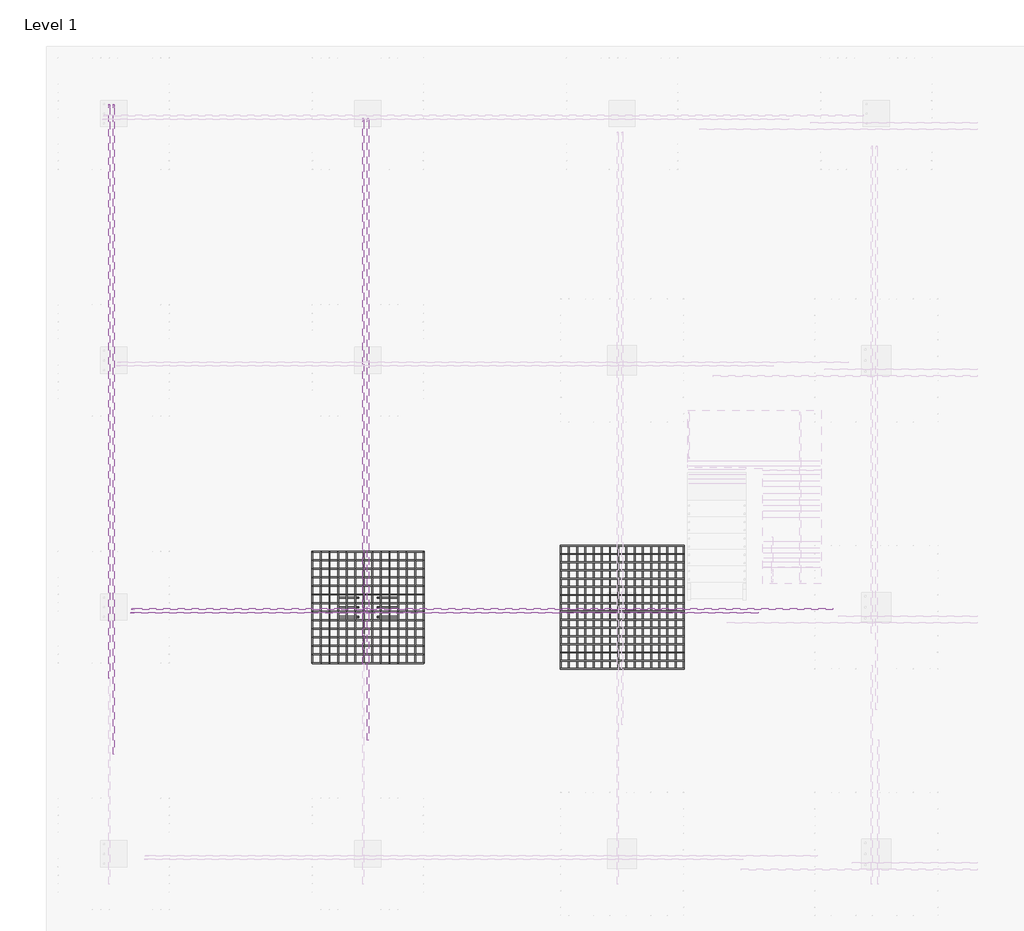
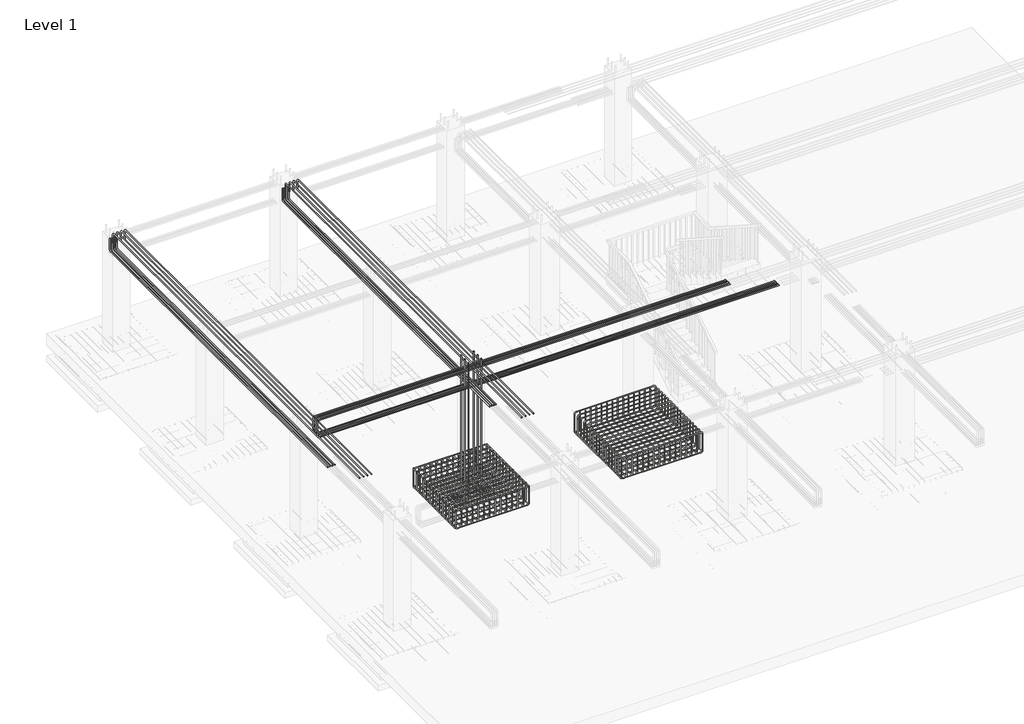
# One storey, part 9 of 17: 21 reinforcing bars.
"""IFC4 building model written with IfcOpenShell, lengths in millimetres."""

from ifc_helpers import new_model, si_unit, point, frame, origin, place, context, project, spatial, polyline, circle_curve, trimmed, segment, composite_curve, source, transform, mapped, element, save
from ifc_brep_helpers import swept_disk

model = new_model("IFC4")

# Units and contexts
model_context = context("Model", 3, world=origin())
ifc_project = project(units=[si_unit("LENGTHUNIT", "METRE", prefix="MILLI")], contexts=[model_context])

# Site, building, storey
site = spatial("IfcSite", under=ifc_project)
building = spatial("IfcBuilding", under=site)
storey = spatial("IfcBuildingStorey", under=building, Name="Level 1", Elevation=0.0)

# Reinforcing bars
placement = place(None, origin())
reinforcing_bar_shape = source(origin(), model_context, "Body", "SolidModel", [
    swept_disk(composite_curve([segment(polyline([(-9341.3632003, 4853.009457, -40.0), (-9341.3632003, 4853.009457, -504.0)]), True, "CONTINUOUS"), segment(trimmed(circle_curve(frame((-9293.3632003, 4853.009457, -504.0), z_axis=(0.0, -1.0, 0.0), x_axis=(-48.0, 0.0, 0.0)), 48.0), [point((-9341.3632003, 4853.009457, -504.0))], [point((-9293.3632003, 4853.009457, -552.0))], True, "CARTESIAN"), True, "CONTINUOUS"), segment(polyline([(-9293.3632003, 4853.009457, -552.0), (-7485.3632003, 4853.009457, -552.0)]), True, "CONTINUOUS"), segment(trimmed(circle_curve(frame((-7485.3632003, 4853.009457, -504.0), z_axis=(0.0, -1.0, 0.0), x_axis=(0.0, 0.0, -48.0)), 48.0), [point((-7485.3632003, 4853.009457, -552.0))], [point((-7437.3632003, 4853.009457, -504.0))], True, "CARTESIAN"), True, "CONTINUOUS"), segment(polyline([(-7437.3632003, 4853.009457, -504.0), (-7437.3632003, 4853.009457, -40.0)]), True, "CONTINUOUS")], self_intersect=False), 8.0),
])
element("IfcReinforcingBar", 1, at=placement, inside=storey, context=model_context, shape_type="MappedRepresentation", body=[
    mapped(reinforcing_bar_shape, transform((0.0, 0.0, 0.0), x_axis=(1.0, 0.0, 0.0), y_axis=(0.0, 1.0, 0.0), z_axis=(0.0, 0.0, 1.0))),
    mapped(reinforcing_bar_shape, transform((0.0, -146.4615385, 0.0), x_axis=(1.0, 0.0, 0.0), y_axis=(0.0, 1.0, 0.0), z_axis=(0.0, 0.0, 1.0))),
    mapped(reinforcing_bar_shape, transform((0.0, -292.9230769, 0.0), x_axis=(1.0, 0.0, 0.0), y_axis=(0.0, 1.0, 0.0), z_axis=(0.0, 0.0, 1.0))),
    mapped(reinforcing_bar_shape, transform((0.0, -439.3846154, 0.0), x_axis=(1.0, 0.0, 0.0), y_axis=(0.0, 1.0, 0.0), z_axis=(0.0, 0.0, 1.0))),
    mapped(reinforcing_bar_shape, transform((0.0, -585.8461538, 0.0), x_axis=(1.0, 0.0, 0.0), y_axis=(0.0, 1.0, 0.0), z_axis=(0.0, 0.0, 1.0))),
    mapped(reinforcing_bar_shape, transform((0.0, -732.3076923, 0.0), x_axis=(1.0, 0.0, 0.0), y_axis=(0.0, 1.0, 0.0), z_axis=(0.0, 0.0, 1.0))),
    mapped(reinforcing_bar_shape, transform((0.0, -878.7692308, 0.0), x_axis=(1.0, 0.0, 0.0), y_axis=(0.0, 1.0, 0.0), z_axis=(0.0, 0.0, 1.0))),
    mapped(reinforcing_bar_shape, transform((0.0, -1025.2307692, 0.0), x_axis=(1.0, 0.0, 0.0), y_axis=(0.0, 1.0, 0.0), z_axis=(0.0, 0.0, 1.0))),
    mapped(reinforcing_bar_shape, transform((0.0, -1171.6923077, 0.0), x_axis=(1.0, 0.0, 0.0), y_axis=(0.0, 1.0, 0.0), z_axis=(0.0, 0.0, 1.0))),
    mapped(reinforcing_bar_shape, transform((0.0, -1318.1538462, 0.0), x_axis=(1.0, 0.0, 0.0), y_axis=(0.0, 1.0, 0.0), z_axis=(0.0, 0.0, 1.0))),
    mapped(reinforcing_bar_shape, transform((0.0, -1464.6153846, 0.0), x_axis=(1.0, 0.0, 0.0), y_axis=(0.0, 1.0, 0.0), z_axis=(0.0, 0.0, 1.0))),
    mapped(reinforcing_bar_shape, transform((0.0, -1611.0769231, 0.0), x_axis=(1.0, 0.0, 0.0), y_axis=(0.0, 1.0, 0.0), z_axis=(0.0, 0.0, 1.0))),
    mapped(reinforcing_bar_shape, transform((0.0, -1757.5384615, 0.0), x_axis=(1.0, 0.0, 0.0), y_axis=(0.0, 1.0, 0.0), z_axis=(0.0, 0.0, 1.0))),
    mapped(reinforcing_bar_shape, transform((0.0, -1904.0, 0.0), x_axis=(1.0, 0.0, 0.0), y_axis=(0.0, 1.0, 0.0), z_axis=(0.0, 0.0, 1.0))),
])
reinforcing_bar_2_shape = source(origin(), model_context, "Body", "SolidModel", [
    swept_disk(composite_curve([segment(polyline([(-9341.3632003, 2949.009457, -504.0), (-9341.3632003, 2949.009457, -96.0)]), True, "CONTINUOUS"), segment(trimmed(circle_curve(frame((-9293.3632003, 2949.009457, -96.0), z_axis=(0.0, 1.0, 0.0), x_axis=(-48.0, 0.0, 0.0)), 48.0), [point((-9341.3632003, 2949.009457, -96.0))], [point((-9293.3632003, 2949.009457, -48.0))], True, "CARTESIAN"), True, "CONTINUOUS"), segment(polyline([(-9293.3632003, 2949.009457, -48.0), (-7485.3632003, 2949.009457, -48.0)]), True, "CONTINUOUS"), segment(trimmed(circle_curve(frame((-7485.3632003, 2949.009457, -96.0), z_axis=(0.0, 1.0, 0.0), x_axis=(0.0, 0.0, 48.0)), 48.0), [point((-7485.3632003, 2949.009457, -48.0))], [point((-7437.3632003, 2949.009457, -96.0))], True, "CARTESIAN"), True, "CONTINUOUS"), segment(polyline([(-7437.3632003, 2949.009457, -96.0), (-7437.3632003, 2949.009457, -504.0)]), True, "CONTINUOUS")], self_intersect=False), 8.0),
])
element("IfcReinforcingBar", 2, at=placement, inside=storey, context=model_context, shape_type="MappedRepresentation", body=[
    mapped(reinforcing_bar_2_shape, transform((0.0, 0.0, 0.0), x_axis=(1.0, 0.0, 0.0), y_axis=(0.0, 1.0, 0.0), z_axis=(0.0, 0.0, 1.0))),
    mapped(reinforcing_bar_2_shape, transform((0.0, 146.4615385, 0.0), x_axis=(1.0, 0.0, 0.0), y_axis=(0.0, 1.0, 0.0), z_axis=(0.0, 0.0, 1.0))),
    mapped(reinforcing_bar_2_shape, transform((0.0, 292.9230769, 0.0), x_axis=(1.0, 0.0, 0.0), y_axis=(0.0, 1.0, 0.0), z_axis=(0.0, 0.0, 1.0))),
    mapped(reinforcing_bar_2_shape, transform((0.0, 439.3846154, 0.0), x_axis=(1.0, 0.0, 0.0), y_axis=(0.0, 1.0, 0.0), z_axis=(0.0, 0.0, 1.0))),
    mapped(reinforcing_bar_2_shape, transform((0.0, 585.8461538, 0.0), x_axis=(1.0, 0.0, 0.0), y_axis=(0.0, 1.0, 0.0), z_axis=(0.0, 0.0, 1.0))),
    mapped(reinforcing_bar_2_shape, transform((0.0, 732.3076923, 0.0), x_axis=(1.0, 0.0, 0.0), y_axis=(0.0, 1.0, 0.0), z_axis=(0.0, 0.0, 1.0))),
    mapped(reinforcing_bar_2_shape, transform((0.0, 878.7692308, 0.0), x_axis=(1.0, 0.0, 0.0), y_axis=(0.0, 1.0, 0.0), z_axis=(0.0, 0.0, 1.0))),
    mapped(reinforcing_bar_2_shape, transform((0.0, 1025.2307692, 0.0), x_axis=(1.0, 0.0, 0.0), y_axis=(0.0, 1.0, 0.0), z_axis=(0.0, 0.0, 1.0))),
    mapped(reinforcing_bar_2_shape, transform((0.0, 1171.6923077, 0.0), x_axis=(1.0, 0.0, 0.0), y_axis=(0.0, 1.0, 0.0), z_axis=(0.0, 0.0, 1.0))),
    mapped(reinforcing_bar_2_shape, transform((0.0, 1318.1538462, 0.0), x_axis=(1.0, 0.0, 0.0), y_axis=(0.0, 1.0, 0.0), z_axis=(0.0, 0.0, 1.0))),
    mapped(reinforcing_bar_2_shape, transform((0.0, 1464.6153846, 0.0), x_axis=(1.0, 0.0, 0.0), y_axis=(0.0, 1.0, 0.0), z_axis=(0.0, 0.0, 1.0))),
    mapped(reinforcing_bar_2_shape, transform((0.0, 1611.0769231, 0.0), x_axis=(1.0, 0.0, 0.0), y_axis=(0.0, 1.0, 0.0), z_axis=(0.0, 0.0, 1.0))),
    mapped(reinforcing_bar_2_shape, transform((0.0, 1757.5384615, 0.0), x_axis=(1.0, 0.0, 0.0), y_axis=(0.0, 1.0, 0.0), z_axis=(0.0, 0.0, 1.0))),
    mapped(reinforcing_bar_2_shape, transform((0.0, 1904.0, 0.0), x_axis=(1.0, 0.0, 0.0), y_axis=(0.0, 1.0, 0.0), z_axis=(0.0, 0.0, 1.0))),
])
reinforcing_bar_3_shape = source(origin(), model_context, "Body", "SolidModel", [
    swept_disk(composite_curve([segment(polyline([(-7437.3632003, 4853.009457, -96.0), (-7437.3632003, 4853.009457, -504.0)]), True, "CONTINUOUS"), segment(trimmed(circle_curve(frame((-7437.3632003, 4805.009457, -504.0), z_axis=(-1.0, 0.0, 0.0), x_axis=(0.0, 48.0, 0.0)), 48.0), [point((-7437.3632003, 4853.009457, -504.0))], [point((-7437.3632003, 4805.009457, -552.0))], True, "CARTESIAN"), True, "CONTINUOUS"), segment(polyline([(-7437.3632003, 4805.009457, -552.0), (-7437.3632003, 2997.009457, -552.0)]), True, "CONTINUOUS"), segment(trimmed(circle_curve(frame((-7437.3632003, 2997.009457, -504.0), z_axis=(-1.0, 0.0, 0.0), x_axis=(0.0, 0.0, -48.0)), 48.0), [point((-7437.3632003, 2997.009457, -552.0))], [point((-7437.3632003, 2949.009457, -504.0))], True, "CARTESIAN"), True, "CONTINUOUS"), segment(polyline([(-7437.3632003, 2949.009457, -504.0), (-7437.3632003, 2949.009457, -96.0)]), True, "CONTINUOUS")], self_intersect=False), 8.0),
])
element("IfcReinforcingBar", 3, at=placement, inside=storey, context=model_context, shape_type="MappedRepresentation", body=[
    mapped(reinforcing_bar_3_shape, transform((0.0, 0.0, 0.0), x_axis=(1.0, 0.0, 0.0), y_axis=(0.0, 1.0, 0.0), z_axis=(0.0, 0.0, 1.0))),
    mapped(reinforcing_bar_3_shape, transform((-146.4615385, 0.0, 0.0), x_axis=(1.0, 0.0, 0.0), y_axis=(0.0, 1.0, 0.0), z_axis=(0.0, 0.0, 1.0))),
    mapped(reinforcing_bar_3_shape, transform((-292.9230769, 0.0, 0.0), x_axis=(1.0, 0.0, 0.0), y_axis=(0.0, 1.0, 0.0), z_axis=(0.0, 0.0, 1.0))),
    mapped(reinforcing_bar_3_shape, transform((-439.3846154, 0.0, 0.0), x_axis=(1.0, 0.0, 0.0), y_axis=(0.0, 1.0, 0.0), z_axis=(0.0, 0.0, 1.0))),
    mapped(reinforcing_bar_3_shape, transform((-585.8461538, 0.0, 0.0), x_axis=(1.0, 0.0, 0.0), y_axis=(0.0, 1.0, 0.0), z_axis=(0.0, 0.0, 1.0))),
    mapped(reinforcing_bar_3_shape, transform((-732.3076923, 0.0, 0.0), x_axis=(1.0, 0.0, 0.0), y_axis=(0.0, 1.0, 0.0), z_axis=(0.0, 0.0, 1.0))),
    mapped(reinforcing_bar_3_shape, transform((-878.7692308, 0.0, 0.0), x_axis=(1.0, 0.0, 0.0), y_axis=(0.0, 1.0, 0.0), z_axis=(0.0, 0.0, 1.0))),
    mapped(reinforcing_bar_3_shape, transform((-1025.2307692, 0.0, 0.0), x_axis=(1.0, 0.0, 0.0), y_axis=(0.0, 1.0, 0.0), z_axis=(0.0, 0.0, 1.0))),
    mapped(reinforcing_bar_3_shape, transform((-1171.6923077, 0.0, 0.0), x_axis=(1.0, 0.0, 0.0), y_axis=(0.0, 1.0, 0.0), z_axis=(0.0, 0.0, 1.0))),
    mapped(reinforcing_bar_3_shape, transform((-1318.1538462, 0.0, 0.0), x_axis=(1.0, 0.0, 0.0), y_axis=(0.0, 1.0, 0.0), z_axis=(0.0, 0.0, 1.0))),
    mapped(reinforcing_bar_3_shape, transform((-1464.6153846, 0.0, 0.0), x_axis=(1.0, 0.0, 0.0), y_axis=(0.0, 1.0, 0.0), z_axis=(0.0, 0.0, 1.0))),
    mapped(reinforcing_bar_3_shape, transform((-1611.0769231, 0.0, 0.0), x_axis=(1.0, 0.0, 0.0), y_axis=(0.0, 1.0, 0.0), z_axis=(0.0, 0.0, 1.0))),
    mapped(reinforcing_bar_3_shape, transform((-1757.5384615, 0.0, 0.0), x_axis=(1.0, 0.0, 0.0), y_axis=(0.0, 1.0, 0.0), z_axis=(0.0, 0.0, 1.0))),
    mapped(reinforcing_bar_3_shape, transform((-1904.0, 0.0, 0.0), x_axis=(1.0, 0.0, 0.0), y_axis=(0.0, 1.0, 0.0), z_axis=(0.0, 0.0, 1.0))),
])
reinforcing_bar_4_shape = source(origin(), model_context, "Body", "SolidModel", [
    swept_disk(composite_curve([segment(polyline([(-9341.3632003, 4853.009457, -504.0), (-9341.3632003, 4853.009457, -96.0)]), True, "CONTINUOUS"), segment(trimmed(circle_curve(frame((-9341.3632003, 4805.009457, -96.0), z_axis=(1.0, 0.0, 0.0), x_axis=(0.0, 48.0, 0.0)), 48.0), [point((-9341.3632003, 4853.009457, -96.0))], [point((-9341.3632003, 4805.009457, -48.0))], True, "CARTESIAN"), True, "CONTINUOUS"), segment(polyline([(-9341.3632003, 4805.009457, -48.0), (-9341.3632003, 2997.009457, -48.0)]), True, "CONTINUOUS"), segment(trimmed(circle_curve(frame((-9341.3632003, 2997.009457, -96.0), z_axis=(1.0, 0.0, 0.0), x_axis=(0.0, 0.0, 48.0)), 48.0), [point((-9341.3632003, 2997.009457, -48.0))], [point((-9341.3632003, 2949.009457, -96.0))], True, "CARTESIAN"), True, "CONTINUOUS"), segment(polyline([(-9341.3632003, 2949.009457, -96.0), (-9341.3632003, 2949.009457, -504.0)]), True, "CONTINUOUS")], self_intersect=False), 8.0),
])
element("IfcReinforcingBar", 4, at=placement, inside=storey, context=model_context, shape_type="MappedRepresentation", body=[
    mapped(reinforcing_bar_4_shape, transform((0.0, 0.0, 0.0), x_axis=(1.0, 0.0, 0.0), y_axis=(0.0, 1.0, 0.0), z_axis=(0.0, 0.0, 1.0))),
    mapped(reinforcing_bar_4_shape, transform((146.4615385, 0.0, 0.0), x_axis=(1.0, 0.0, 0.0), y_axis=(0.0, 1.0, 0.0), z_axis=(0.0, 0.0, 1.0))),
    mapped(reinforcing_bar_4_shape, transform((292.9230769, 0.0, 0.0), x_axis=(1.0, 0.0, 0.0), y_axis=(0.0, 1.0, 0.0), z_axis=(0.0, 0.0, 1.0))),
    mapped(reinforcing_bar_4_shape, transform((439.3846154, 0.0, 0.0), x_axis=(1.0, 0.0, 0.0), y_axis=(0.0, 1.0, 0.0), z_axis=(0.0, 0.0, 1.0))),
    mapped(reinforcing_bar_4_shape, transform((585.8461538, 0.0, 0.0), x_axis=(1.0, 0.0, 0.0), y_axis=(0.0, 1.0, 0.0), z_axis=(0.0, 0.0, 1.0))),
    mapped(reinforcing_bar_4_shape, transform((732.3076923, 0.0, 0.0), x_axis=(1.0, 0.0, 0.0), y_axis=(0.0, 1.0, 0.0), z_axis=(0.0, 0.0, 1.0))),
    mapped(reinforcing_bar_4_shape, transform((878.7692308, 0.0, 0.0), x_axis=(1.0, 0.0, 0.0), y_axis=(0.0, 1.0, 0.0), z_axis=(0.0, 0.0, 1.0))),
    mapped(reinforcing_bar_4_shape, transform((1025.2307692, 0.0, 0.0), x_axis=(1.0, 0.0, 0.0), y_axis=(0.0, 1.0, 0.0), z_axis=(0.0, 0.0, 1.0))),
    mapped(reinforcing_bar_4_shape, transform((1171.6923077, 0.0, 0.0), x_axis=(1.0, 0.0, 0.0), y_axis=(0.0, 1.0, 0.0), z_axis=(0.0, 0.0, 1.0))),
    mapped(reinforcing_bar_4_shape, transform((1318.1538462, 0.0, 0.0), x_axis=(1.0, 0.0, 0.0), y_axis=(0.0, 1.0, 0.0), z_axis=(0.0, 0.0, 1.0))),
    mapped(reinforcing_bar_4_shape, transform((1464.6153846, 0.0, 0.0), x_axis=(1.0, 0.0, 0.0), y_axis=(0.0, 1.0, 0.0), z_axis=(0.0, 0.0, 1.0))),
    mapped(reinforcing_bar_4_shape, transform((1611.0769231, 0.0, 0.0), x_axis=(1.0, 0.0, 0.0), y_axis=(0.0, 1.0, 0.0), z_axis=(0.0, 0.0, 1.0))),
    mapped(reinforcing_bar_4_shape, transform((1757.5384615, 0.0, 0.0), x_axis=(1.0, 0.0, 0.0), y_axis=(0.0, 1.0, 0.0), z_axis=(0.0, 0.0, 1.0))),
    mapped(reinforcing_bar_4_shape, transform((1904.0, 0.0, 0.0), x_axis=(1.0, 0.0, 0.0), y_axis=(0.0, 1.0, 0.0), z_axis=(0.0, 0.0, 1.0))),
])
reinforcing_bar_5_shape = source(origin(), model_context, "Body", "SolidModel", [
    swept_disk(composite_curve([segment(polyline([(-8901.9785849, 4066.509457, -550.0), (-8604.8632003, 4066.509457, -550.0)]), True, "CONTINUOUS"), segment(trimmed(circle_curve(frame((-8604.8632003, 4066.509457, -500.0), z_axis=(0.0, -1.0, 0.0), x_axis=(0.0, 0.0, -50.0)), 50.0), [point((-8604.8632003, 4066.509457, -550.0))], [point((-8554.8632003, 4066.509457, -500.0))], True, "CARTESIAN"), True, "CONTINUOUS"), segment(polyline([(-8554.8632003, 4066.509457, -500.0), (-8554.8632003, 4066.509457, 3260.0)]), True, "CONTINUOUS")], self_intersect=False), 10.0),
])
element("IfcReinforcingBar", 5, at=placement, inside=storey, context=model_context, shape_type="MappedRepresentation", body=[
    mapped(reinforcing_bar_5_shape, transform((0.0, 0.0, 0.0), x_axis=(1.0, 0.0, 0.0), y_axis=(0.0, 1.0, 0.0), z_axis=(0.0, 0.0, 1.0))),
    mapped(reinforcing_bar_5_shape, transform((0.0, -165.5, 0.0), x_axis=(1.0, 0.0, 0.0), y_axis=(0.0, 1.0, 0.0), z_axis=(0.0, 0.0, 1.0))),
    mapped(reinforcing_bar_5_shape, transform((0.0, -331.0, 0.0), x_axis=(1.0, 0.0, 0.0), y_axis=(0.0, 1.0, 0.0), z_axis=(0.0, 0.0, 1.0))),
])
reinforcing_bar_6_shape = source(origin(), model_context, "Body", "SolidModel", [
    swept_disk(composite_curve([segment(polyline([(-7876.7478157, 3735.509457, -550.0), (-8173.8632003, 3735.509457, -550.0)]), True, "CONTINUOUS"), segment(trimmed(circle_curve(frame((-8173.8632003, 3735.509457, -500.0), z_axis=(0.0, 1.0, 0.0), x_axis=(0.0, 0.0, -50.0)), 50.0), [point((-8173.8632003, 3735.509457, -550.0))], [point((-8223.8632003, 3735.509457, -500.0))], True, "CARTESIAN"), True, "CONTINUOUS"), segment(polyline([(-8223.8632003, 3735.509457, -500.0), (-8223.8632003, 3735.509457, 3260.0)]), True, "CONTINUOUS")], self_intersect=False), 10.0),
])
element("IfcReinforcingBar", 6, at=placement, inside=storey, context=model_context, shape_type="MappedRepresentation", body=[
    mapped(reinforcing_bar_6_shape, transform((0.0, 0.0, 0.0), x_axis=(1.0, 0.0, 0.0), y_axis=(0.0, 1.0, 0.0), z_axis=(0.0, 0.0, 1.0))),
    mapped(reinforcing_bar_6_shape, transform((0.0, 165.5, 0.0), x_axis=(1.0, 0.0, 0.0), y_axis=(0.0, 1.0, 0.0), z_axis=(0.0, 0.0, 1.0))),
    mapped(reinforcing_bar_6_shape, transform((0.0, 331.0, 0.0), x_axis=(1.0, 0.0, 0.0), y_axis=(0.0, 1.0, 0.0), z_axis=(0.0, 0.0, 1.0))),
])
reinforcing_bar_7_shape = source(origin(), model_context, "Body", "SolidModel", [
    swept_disk(composite_curve([segment(polyline([(-5096.3632003, 4953.009457, -140.0), (-5096.3632003, 4953.009457, -554.0)]), True, "CONTINUOUS"), segment(trimmed(circle_curve(frame((-5048.3632003, 4953.009457, -554.0), z_axis=(0.0, -1.0, 0.0), x_axis=(-48.0, 0.0, 0.0)), 48.0), [point((-5096.3632003, 4953.009457, -554.0))], [point((-5048.3632003, 4953.009457, -602.0))], True, "CARTESIAN"), True, "CONTINUOUS"), segment(polyline([(-5048.3632003, 4953.009457, -602.0), (-3040.3632003, 4953.009457, -602.0)]), True, "CONTINUOUS"), segment(trimmed(circle_curve(frame((-3040.3632003, 4953.009457, -554.0), z_axis=(0.0, -1.0, 0.0), x_axis=(0.0, 0.0, -48.0)), 48.0), [point((-3040.3632003, 4953.009457, -602.0))], [point((-2992.3632003, 4953.009457, -554.0))], True, "CARTESIAN"), True, "CONTINUOUS"), segment(polyline([(-2992.3632003, 4953.009457, -554.0), (-2992.3632003, 4953.009457, -140.0)]), True, "CONTINUOUS")], self_intersect=False), 8.0),
])
element("IfcReinforcingBar", 7, at=placement, inside=storey, context=model_context, shape_type="MappedRepresentation", body=[
    mapped(reinforcing_bar_7_shape, transform((0.0, 0.0, 0.0), x_axis=(1.0, 0.0, 0.0), y_axis=(0.0, 1.0, 0.0), z_axis=(0.0, 0.0, 1.0))),
    mapped(reinforcing_bar_7_shape, transform((0.0, -140.2666667, 0.0), x_axis=(1.0, 0.0, 0.0), y_axis=(0.0, 1.0, 0.0), z_axis=(0.0, 0.0, 1.0))),
    mapped(reinforcing_bar_7_shape, transform((0.0, -280.5333333, 0.0), x_axis=(1.0, 0.0, 0.0), y_axis=(0.0, 1.0, 0.0), z_axis=(0.0, 0.0, 1.0))),
    mapped(reinforcing_bar_7_shape, transform((0.0, -420.8, 0.0), x_axis=(1.0, 0.0, 0.0), y_axis=(0.0, 1.0, 0.0), z_axis=(0.0, 0.0, 1.0))),
    mapped(reinforcing_bar_7_shape, transform((0.0, -561.0666667, 0.0), x_axis=(1.0, 0.0, 0.0), y_axis=(0.0, 1.0, 0.0), z_axis=(0.0, 0.0, 1.0))),
    mapped(reinforcing_bar_7_shape, transform((0.0, -701.3333333, 0.0), x_axis=(1.0, 0.0, 0.0), y_axis=(0.0, 1.0, 0.0), z_axis=(0.0, 0.0, 1.0))),
    mapped(reinforcing_bar_7_shape, transform((0.0, -841.6, 0.0), x_axis=(1.0, 0.0, 0.0), y_axis=(0.0, 1.0, 0.0), z_axis=(0.0, 0.0, 1.0))),
    mapped(reinforcing_bar_7_shape, transform((0.0, -981.8666667, 0.0), x_axis=(1.0, 0.0, 0.0), y_axis=(0.0, 1.0, 0.0), z_axis=(0.0, 0.0, 1.0))),
    mapped(reinforcing_bar_7_shape, transform((0.0, -1122.1333333, 0.0), x_axis=(1.0, 0.0, 0.0), y_axis=(0.0, 1.0, 0.0), z_axis=(0.0, 0.0, 1.0))),
    mapped(reinforcing_bar_7_shape, transform((0.0, -1262.4, 0.0), x_axis=(1.0, 0.0, 0.0), y_axis=(0.0, 1.0, 0.0), z_axis=(0.0, 0.0, 1.0))),
    mapped(reinforcing_bar_7_shape, transform((0.0, -1402.6666667, 0.0), x_axis=(1.0, 0.0, 0.0), y_axis=(0.0, 1.0, 0.0), z_axis=(0.0, 0.0, 1.0))),
    mapped(reinforcing_bar_7_shape, transform((0.0, -1542.9333333, 0.0), x_axis=(1.0, 0.0, 0.0), y_axis=(0.0, 1.0, 0.0), z_axis=(0.0, 0.0, 1.0))),
    mapped(reinforcing_bar_7_shape, transform((0.0, -1683.2, 0.0), x_axis=(1.0, 0.0, 0.0), y_axis=(0.0, 1.0, 0.0), z_axis=(0.0, 0.0, 1.0))),
    mapped(reinforcing_bar_7_shape, transform((0.0, -1823.4666667, 0.0), x_axis=(1.0, 0.0, 0.0), y_axis=(0.0, 1.0, 0.0), z_axis=(0.0, 0.0, 1.0))),
    mapped(reinforcing_bar_7_shape, transform((0.0, -1963.7333333, 0.0), x_axis=(1.0, 0.0, 0.0), y_axis=(0.0, 1.0, 0.0), z_axis=(0.0, 0.0, 1.0))),
    mapped(reinforcing_bar_7_shape, transform((0.0, -2104.0, 0.0), x_axis=(1.0, 0.0, 0.0), y_axis=(0.0, 1.0, 0.0), z_axis=(0.0, 0.0, 1.0))),
])
reinforcing_bar_8_shape = source(origin(), model_context, "Body", "SolidModel", [
    swept_disk(composite_curve([segment(polyline([(-5096.3632003, 2849.009457, -554.0), (-5096.3632003, 2849.009457, -96.0)]), True, "CONTINUOUS"), segment(trimmed(circle_curve(frame((-5048.3632003, 2849.009457, -96.0), z_axis=(0.0, 1.0, 0.0), x_axis=(-48.0, 0.0, 0.0)), 48.0), [point((-5096.3632003, 2849.009457, -96.0))], [point((-5048.3632003, 2849.009457, -48.0))], True, "CARTESIAN"), True, "CONTINUOUS"), segment(polyline([(-5048.3632003, 2849.009457, -48.0), (-3040.3632003, 2849.009457, -48.0)]), True, "CONTINUOUS"), segment(trimmed(circle_curve(frame((-3040.3632003, 2849.009457, -96.0), z_axis=(0.0, 1.0, 0.0), x_axis=(0.0, 0.0, 48.0)), 48.0), [point((-3040.3632003, 2849.009457, -48.0))], [point((-2992.3632003, 2849.009457, -96.0))], True, "CARTESIAN"), True, "CONTINUOUS"), segment(polyline([(-2992.3632003, 2849.009457, -96.0), (-2992.3632003, 2849.009457, -554.0)]), True, "CONTINUOUS")], self_intersect=False), 8.0),
])
element("IfcReinforcingBar", 8, at=placement, inside=storey, context=model_context, shape_type="MappedRepresentation", body=[
    mapped(reinforcing_bar_8_shape, transform((0.0, 0.0, 0.0), x_axis=(1.0, 0.0, 0.0), y_axis=(0.0, 1.0, 0.0), z_axis=(0.0, 0.0, 1.0))),
    mapped(reinforcing_bar_8_shape, transform((0.0, 140.2666667, 0.0), x_axis=(1.0, 0.0, 0.0), y_axis=(0.0, 1.0, 0.0), z_axis=(0.0, 0.0, 1.0))),
    mapped(reinforcing_bar_8_shape, transform((0.0, 280.5333333, 0.0), x_axis=(1.0, 0.0, 0.0), y_axis=(0.0, 1.0, 0.0), z_axis=(0.0, 0.0, 1.0))),
    mapped(reinforcing_bar_8_shape, transform((0.0, 420.8, 0.0), x_axis=(1.0, 0.0, 0.0), y_axis=(0.0, 1.0, 0.0), z_axis=(0.0, 0.0, 1.0))),
    mapped(reinforcing_bar_8_shape, transform((0.0, 561.0666667, 0.0), x_axis=(1.0, 0.0, 0.0), y_axis=(0.0, 1.0, 0.0), z_axis=(0.0, 0.0, 1.0))),
    mapped(reinforcing_bar_8_shape, transform((0.0, 701.3333333, 0.0), x_axis=(1.0, 0.0, 0.0), y_axis=(0.0, 1.0, 0.0), z_axis=(0.0, 0.0, 1.0))),
    mapped(reinforcing_bar_8_shape, transform((0.0, 841.6, 0.0), x_axis=(1.0, 0.0, 0.0), y_axis=(0.0, 1.0, 0.0), z_axis=(0.0, 0.0, 1.0))),
    mapped(reinforcing_bar_8_shape, transform((0.0, 981.8666667, 0.0), x_axis=(1.0, 0.0, 0.0), y_axis=(0.0, 1.0, 0.0), z_axis=(0.0, 0.0, 1.0))),
    mapped(reinforcing_bar_8_shape, transform((0.0, 1122.1333333, 0.0), x_axis=(1.0, 0.0, 0.0), y_axis=(0.0, 1.0, 0.0), z_axis=(0.0, 0.0, 1.0))),
    mapped(reinforcing_bar_8_shape, transform((0.0, 1262.4, 0.0), x_axis=(1.0, 0.0, 0.0), y_axis=(0.0, 1.0, 0.0), z_axis=(0.0, 0.0, 1.0))),
    mapped(reinforcing_bar_8_shape, transform((0.0, 1402.6666667, 0.0), x_axis=(1.0, 0.0, 0.0), y_axis=(0.0, 1.0, 0.0), z_axis=(0.0, 0.0, 1.0))),
    mapped(reinforcing_bar_8_shape, transform((0.0, 1542.9333333, 0.0), x_axis=(1.0, 0.0, 0.0), y_axis=(0.0, 1.0, 0.0), z_axis=(0.0, 0.0, 1.0))),
    mapped(reinforcing_bar_8_shape, transform((0.0, 1683.2, 0.0), x_axis=(1.0, 0.0, 0.0), y_axis=(0.0, 1.0, 0.0), z_axis=(0.0, 0.0, 1.0))),
    mapped(reinforcing_bar_8_shape, transform((0.0, 1823.4666667, 0.0), x_axis=(1.0, 0.0, 0.0), y_axis=(0.0, 1.0, 0.0), z_axis=(0.0, 0.0, 1.0))),
    mapped(reinforcing_bar_8_shape, transform((0.0, 1963.7333333, 0.0), x_axis=(1.0, 0.0, 0.0), y_axis=(0.0, 1.0, 0.0), z_axis=(0.0, 0.0, 1.0))),
    mapped(reinforcing_bar_8_shape, transform((0.0, 2104.0, 0.0), x_axis=(1.0, 0.0, 0.0), y_axis=(0.0, 1.0, 0.0), z_axis=(0.0, 0.0, 1.0))),
])
reinforcing_bar_9_shape = source(origin(), model_context, "Body", "SolidModel", [
    swept_disk(composite_curve([segment(polyline([(-2992.3632003, 4953.009457, -100.0), (-2992.3632003, 4953.009457, -554.0)]), True, "CONTINUOUS"), segment(trimmed(circle_curve(frame((-2992.3632003, 4905.009457, -554.0), z_axis=(-1.0, 0.0, 0.0), x_axis=(0.0, 48.0, 0.0)), 48.0), [point((-2992.3632003, 4953.009457, -554.0))], [point((-2992.3632003, 4905.009457, -602.0))], True, "CARTESIAN"), True, "CONTINUOUS"), segment(polyline([(-2992.3632003, 4905.009457, -602.0), (-2992.3632003, 2897.009457, -602.0)]), True, "CONTINUOUS"), segment(trimmed(circle_curve(frame((-2992.3632003, 2897.009457, -554.0), z_axis=(-1.0, 0.0, 0.0), x_axis=(0.0, 0.0, -48.0)), 48.0), [point((-2992.3632003, 2897.009457, -602.0))], [point((-2992.3632003, 2849.009457, -554.0))], True, "CARTESIAN"), True, "CONTINUOUS"), segment(polyline([(-2992.3632003, 2849.009457, -554.0), (-2992.3632003, 2849.009457, -100.0)]), True, "CONTINUOUS")], self_intersect=False), 8.0),
])
element("IfcReinforcingBar", 9, at=placement, inside=storey, context=model_context, shape_type="MappedRepresentation", body=[
    mapped(reinforcing_bar_9_shape, transform((0.0, 0.0, 0.0), x_axis=(1.0, 0.0, 0.0), y_axis=(0.0, 1.0, 0.0), z_axis=(0.0, 0.0, 1.0))),
    mapped(reinforcing_bar_9_shape, transform((-140.2666667, 0.0, 0.0), x_axis=(1.0, 0.0, 0.0), y_axis=(0.0, 1.0, 0.0), z_axis=(0.0, 0.0, 1.0))),
    mapped(reinforcing_bar_9_shape, transform((-280.5333333, 0.0, 0.0), x_axis=(1.0, 0.0, 0.0), y_axis=(0.0, 1.0, 0.0), z_axis=(0.0, 0.0, 1.0))),
    mapped(reinforcing_bar_9_shape, transform((-420.8, 0.0, 0.0), x_axis=(1.0, 0.0, 0.0), y_axis=(0.0, 1.0, 0.0), z_axis=(0.0, 0.0, 1.0))),
    mapped(reinforcing_bar_9_shape, transform((-561.0666667, 0.0, 0.0), x_axis=(1.0, 0.0, 0.0), y_axis=(0.0, 1.0, 0.0), z_axis=(0.0, 0.0, 1.0))),
    mapped(reinforcing_bar_9_shape, transform((-701.3333333, 0.0, 0.0), x_axis=(1.0, 0.0, 0.0), y_axis=(0.0, 1.0, 0.0), z_axis=(0.0, 0.0, 1.0))),
    mapped(reinforcing_bar_9_shape, transform((-841.6, 0.0, 0.0), x_axis=(1.0, 0.0, 0.0), y_axis=(0.0, 1.0, 0.0), z_axis=(0.0, 0.0, 1.0))),
    mapped(reinforcing_bar_9_shape, transform((-981.8666667, 0.0, 0.0), x_axis=(1.0, 0.0, 0.0), y_axis=(0.0, 1.0, 0.0), z_axis=(0.0, 0.0, 1.0))),
    mapped(reinforcing_bar_9_shape, transform((-1122.1333333, 0.0, 0.0), x_axis=(1.0, 0.0, 0.0), y_axis=(0.0, 1.0, 0.0), z_axis=(0.0, 0.0, 1.0))),
    mapped(reinforcing_bar_9_shape, transform((-1262.4, 0.0, 0.0), x_axis=(1.0, 0.0, 0.0), y_axis=(0.0, 1.0, 0.0), z_axis=(0.0, 0.0, 1.0))),
    mapped(reinforcing_bar_9_shape, transform((-1402.6666667, 0.0, 0.0), x_axis=(1.0, 0.0, 0.0), y_axis=(0.0, 1.0, 0.0), z_axis=(0.0, 0.0, 1.0))),
    mapped(reinforcing_bar_9_shape, transform((-1542.9333333, 0.0, 0.0), x_axis=(1.0, 0.0, 0.0), y_axis=(0.0, 1.0, 0.0), z_axis=(0.0, 0.0, 1.0))),
    mapped(reinforcing_bar_9_shape, transform((-1683.2, 0.0, 0.0), x_axis=(1.0, 0.0, 0.0), y_axis=(0.0, 1.0, 0.0), z_axis=(0.0, 0.0, 1.0))),
    mapped(reinforcing_bar_9_shape, transform((-1823.4666667, 0.0, 0.0), x_axis=(1.0, 0.0, 0.0), y_axis=(0.0, 1.0, 0.0), z_axis=(0.0, 0.0, 1.0))),
    mapped(reinforcing_bar_9_shape, transform((-1963.7333333, 0.0, 0.0), x_axis=(1.0, 0.0, 0.0), y_axis=(0.0, 1.0, 0.0), z_axis=(0.0, 0.0, 1.0))),
    mapped(reinforcing_bar_9_shape, transform((-2104.0, 0.0, 0.0), x_axis=(1.0, 0.0, 0.0), y_axis=(0.0, 1.0, 0.0), z_axis=(0.0, 0.0, 1.0))),
])
reinforcing_bar_10_shape = source(origin(), model_context, "Body", "SolidModel", [
    swept_disk(composite_curve([segment(polyline([(-449.7632003, 3810.509457, 2507.5), (-12374.4632003, 3810.509457, 2507.5)]), True, "CONTINUOUS"), segment(trimmed(circle_curve(frame((-12374.4632003, 3810.509457, 2557.5), z_axis=(0.0, 1.0, 0.0), x_axis=(0.0, 0.0, -50.0)), 50.0), [point((-12374.4632003, 3810.509457, 2507.5))], [point((-12424.4632003, 3810.509457, 2557.5))], True, "CARTESIAN"), True, "CONTINUOUS"), segment(polyline([(-12424.4632003, 3810.509457, 2557.5), (-12424.4632003, 3810.509457, 2707.4)]), True, "CONTINUOUS")], self_intersect=False), 10.0),
])
element("IfcReinforcingBar", 10, at=placement, inside=storey, context=model_context, shape_type="MappedRepresentation", body=[
    mapped(reinforcing_bar_10_shape, transform((0.0, 0.0, 0.0), x_axis=(1.0, 0.0, 0.0), y_axis=(0.0, 1.0, 0.0), z_axis=(0.0, 0.0, 1.0))),
    mapped(reinforcing_bar_10_shape, transform((0.0, 60.3333333, 0.0), x_axis=(1.0, 0.0, 0.0), y_axis=(0.0, 1.0, 0.0), z_axis=(0.0, 0.0, 1.0))),
    mapped(reinforcing_bar_10_shape, transform((0.0, 120.6666667, 0.0), x_axis=(1.0, 0.0, 0.0), y_axis=(0.0, 1.0, 0.0), z_axis=(0.0, 0.0, 1.0))),
    mapped(reinforcing_bar_10_shape, transform((0.0, 181.0, 0.0), x_axis=(1.0, 0.0, 0.0), y_axis=(0.0, 1.0, 0.0), z_axis=(0.0, 0.0, 1.0))),
])
reinforcing_bar_11_shape = source(origin(), model_context, "Body", "SolidModel", [
    swept_disk(composite_curve([segment(polyline([(-1724.7632003, 3991.509457, 2988.5), (-12389.2132003, 3991.509457, 2988.5)]), True, "CONTINUOUS"), segment(trimmed(circle_curve(frame((-12389.2132003, 3991.509457, 2938.5), z_axis=(0.0, -1.0, 0.0), x_axis=(0.0, 0.0, 50.0)), 50.0), [point((-12389.2132003, 3991.509457, 2988.5))], [point((-12439.2132003, 3991.509457, 2938.5))], True, "CARTESIAN"), True, "CONTINUOUS"), segment(polyline([(-12439.2132003, 3991.509457, 2938.5), (-12439.2132003, 3991.509457, 2648.0)]), True, "CONTINUOUS")], self_intersect=False), 10.0),
])
element("IfcReinforcingBar", 11, at=placement, inside=storey, context=model_context, shape_type="MappedRepresentation", body=[
    mapped(reinforcing_bar_11_shape, transform((0.0, 0.0, 0.0), x_axis=(1.0, 0.0, 0.0), y_axis=(0.0, 1.0, 0.0), z_axis=(0.0, 0.0, 1.0))),
    mapped(reinforcing_bar_11_shape, transform((0.0, -60.3333333, 0.0), x_axis=(1.0, 0.0, 0.0), y_axis=(0.0, 1.0, 0.0), z_axis=(0.0, 0.0, 1.0))),
    mapped(reinforcing_bar_11_shape, transform((0.0, -120.6666667, 0.0), x_axis=(1.0, 0.0, 0.0), y_axis=(0.0, 1.0, 0.0), z_axis=(0.0, 0.0, 1.0))),
    mapped(reinforcing_bar_11_shape, transform((0.0, -181.0, 0.0), x_axis=(1.0, 0.0, 0.0), y_axis=(0.0, 1.0, 0.0), z_axis=(0.0, 0.0, 1.0))),
])
reinforcing_bar_12_shape = source(origin(), model_context, "Body", "SolidModel", [
    swept_disk(composite_curve([segment(polyline([(-12634.3632003, 12490.509457, 2855.325), (-12634.3632003, 12490.509457, 2568.0)]), True, "CONTINUOUS"), segment(trimmed(circle_curve(frame((-12634.3632003, 12440.509457, 2568.0), z_axis=(-1.0, 0.0, 0.0), x_axis=(0.0, 50.0, 0.0)), 50.0), [point((-12634.3632003, 12490.509457, 2568.0))], [point((-12634.3632003, 12440.509457, 2518.0))], True, "CARTESIAN"), True, "CONTINUOUS"), segment(polyline([(-12634.3632003, 12440.509457, 2518.0), (-12634.3632003, 2690.509457, 2518.0)]), True, "CONTINUOUS")], self_intersect=False), 10.0),
])
element("IfcReinforcingBar", 12, at=placement, inside=storey, context=model_context, shape_type="MappedRepresentation", body=[
    mapped(reinforcing_bar_12_shape, transform((0.0, 0.0, 0.0), x_axis=(1.0, 0.0, 0.0), y_axis=(0.0, 1.0, 0.0), z_axis=(0.0, 0.0, 1.0))),
    mapped(reinforcing_bar_12_shape, transform((-60.0, 0.0, 0.0), x_axis=(1.0, 0.0, 0.0), y_axis=(0.0, 1.0, 0.0), z_axis=(0.0, 0.0, 1.0))),
    mapped(reinforcing_bar_12_shape, transform((-120.0, 0.0, 0.0), x_axis=(1.0, 0.0, 0.0), y_axis=(0.0, 1.0, 0.0), z_axis=(0.0, 0.0, 1.0))),
    mapped(reinforcing_bar_12_shape, transform((-180.0, 0.0, 0.0), x_axis=(1.0, 0.0, 0.0), y_axis=(0.0, 1.0, 0.0), z_axis=(0.0, 0.0, 1.0))),
])
reinforcing_bar_13_shape = source(origin(), model_context, "Body", "SolidModel", [
    swept_disk(composite_curve([segment(polyline([(-12734.3632003, 12490.509457, 2707.4), (-12734.3632003, 12490.509457, 2928.0)]), True, "CONTINUOUS"), segment(trimmed(circle_curve(frame((-12734.3632003, 12440.509457, 2928.0), z_axis=(1.0, 0.0, 0.0), x_axis=(0.0, 50.0, 0.0)), 50.0), [point((-12734.3632003, 12490.509457, 2928.0))], [point((-12734.3632003, 12440.509457, 2978.0))], True, "CARTESIAN"), True, "CONTINUOUS"), segment(polyline([(-12734.3632003, 12440.509457, 2978.0), (-12734.3632003, 1390.509457, 2978.0)]), True, "CONTINUOUS")], self_intersect=False), 10.0),
])
element("IfcReinforcingBar", 13, at=placement, inside=storey, context=model_context, shape_type="MappedRepresentation", body=[
    mapped(reinforcing_bar_13_shape, transform((0.0, 0.0, 0.0), x_axis=(1.0, 0.0, 0.0), y_axis=(0.0, 1.0, 0.0), z_axis=(0.0, 0.0, 1.0))),
    mapped(reinforcing_bar_13_shape, transform((101.6, 0.0, 0.0), x_axis=(1.0, 0.0, 0.0), y_axis=(0.0, 1.0, 0.0), z_axis=(0.0, 0.0, 1.0))),
    mapped(reinforcing_bar_13_shape, transform((203.2, 0.0, 0.0), x_axis=(1.0, 0.0, 0.0), y_axis=(0.0, 1.0, 0.0), z_axis=(0.0, 0.0, 1.0))),
    mapped(reinforcing_bar_13_shape, transform((304.8, 0.0, 0.0), x_axis=(1.0, 0.0, 0.0), y_axis=(0.0, 1.0, 0.0), z_axis=(0.0, 0.0, 1.0))),
])
reinforcing_bar_14_shape = source(origin(), model_context, "Body", "SolidModel", [
    swept_disk(composite_curve([segment(polyline([(-8309.3632003, 12252.809457, 2855.325), (-8309.3632003, 12252.809457, 2568.0)]), True, "CONTINUOUS"), segment(trimmed(circle_curve(frame((-8309.3632003, 12202.809457, 2568.0), z_axis=(-1.0, 0.0, 0.0), x_axis=(0.0, 50.0, 0.0)), 50.0), [point((-8309.3632003, 12252.809457, 2568.0))], [point((-8309.3632003, 12202.809457, 2518.0))], True, "CARTESIAN"), True, "CONTINUOUS"), segment(polyline([(-8309.3632003, 12202.809457, 2518.0), (-8309.3632003, 2928.209457, 2518.0)]), True, "CONTINUOUS")], self_intersect=False), 10.0),
])
element("IfcReinforcingBar", 14, at=placement, inside=storey, context=model_context, shape_type="MappedRepresentation", body=[
    mapped(reinforcing_bar_14_shape, transform((0.0, 0.0, 0.0), x_axis=(1.0, 0.0, 0.0), y_axis=(0.0, 1.0, 0.0), z_axis=(0.0, 0.0, 1.0))),
    mapped(reinforcing_bar_14_shape, transform((-53.3333333, 0.0, 0.0), x_axis=(1.0, 0.0, 0.0), y_axis=(0.0, 1.0, 0.0), z_axis=(0.0, 0.0, 1.0))),
    mapped(reinforcing_bar_14_shape, transform((-106.6666667, 0.0, 0.0), x_axis=(1.0, 0.0, 0.0), y_axis=(0.0, 1.0, 0.0), z_axis=(0.0, 0.0, 1.0))),
    mapped(reinforcing_bar_14_shape, transform((-160.0, 0.0, 0.0), x_axis=(1.0, 0.0, 0.0), y_axis=(0.0, 1.0, 0.0), z_axis=(0.0, 0.0, 1.0))),
])
reinforcing_bar_15_shape = source(origin(), model_context, "Body", "SolidModel", [
    swept_disk(composite_curve([segment(polyline([(-8389.3632003, 12252.809457, 2707.4), (-8389.3632003, 12252.809457, 2928.0)]), True, "CONTINUOUS"), segment(trimmed(circle_curve(frame((-8389.3632003, 12202.809457, 2928.0), z_axis=(1.0, 0.0, 0.0), x_axis=(0.0, 50.0, 0.0)), 50.0), [point((-8389.3632003, 12252.809457, 2928.0))], [point((-8389.3632003, 12202.809457, 2978.0))], True, "CARTESIAN"), True, "CONTINUOUS"), segment(polyline([(-8389.3632003, 12202.809457, 2978.0), (-8389.3632003, 1628.209457, 2978.0)]), True, "CONTINUOUS")], self_intersect=False), 10.0),
])
element("IfcReinforcingBar", 15, at=placement, inside=storey, context=model_context, shape_type="MappedRepresentation", body=[
    mapped(reinforcing_bar_15_shape, transform((0.0, 0.0, 0.0), x_axis=(1.0, 0.0, 0.0), y_axis=(0.0, 1.0, 0.0), z_axis=(0.0, 0.0, 1.0))),
    mapped(reinforcing_bar_15_shape, transform((101.6, 0.0, 0.0), x_axis=(1.0, 0.0, 0.0), y_axis=(0.0, 1.0, 0.0), z_axis=(0.0, 0.0, 1.0))),
    mapped(reinforcing_bar_15_shape, transform((203.2, 0.0, 0.0), x_axis=(1.0, 0.0, 0.0), y_axis=(0.0, 1.0, 0.0), z_axis=(0.0, 0.0, 1.0))),
    mapped(reinforcing_bar_15_shape, transform((304.8, 0.0, 0.0), x_axis=(1.0, 0.0, 0.0), y_axis=(0.0, 1.0, 0.0), z_axis=(0.0, 0.0, 1.0))),
])
reinforcing_bar_16_shape = source(origin(), model_context, "Body", "SolidModel", [
    swept_disk(composite_curve([segment(polyline([(-449.7632003, 3810.509457, 2507.5), (-12374.4632003, 3810.509457, 2507.5)]), True, "CONTINUOUS"), segment(trimmed(circle_curve(frame((-12374.4632003, 3810.509457, 2557.5), z_axis=(0.0, 1.0, 0.0), x_axis=(0.0, 0.0, -50.0)), 50.0), [point((-12374.4632003, 3810.509457, 2507.5))], [point((-12424.4632003, 3810.509457, 2557.5))], True, "CARTESIAN"), True, "CONTINUOUS"), segment(polyline([(-12424.4632003, 3810.509457, 2557.5), (-12424.4632003, 3810.509457, 2707.4)]), True, "CONTINUOUS")], self_intersect=False), 10.0),
])
element("IfcReinforcingBar", 16, at=placement, inside=storey, context=model_context, shape_type="MappedRepresentation", body=[
    mapped(reinforcing_bar_16_shape, transform((0.0, 0.0, 0.0), x_axis=(1.0, 0.0, 0.0), y_axis=(0.0, 1.0, 0.0), z_axis=(0.0, 0.0, 1.0))),
    mapped(reinforcing_bar_16_shape, transform((0.0, 60.3333333, 0.0), x_axis=(1.0, 0.0, 0.0), y_axis=(0.0, 1.0, 0.0), z_axis=(0.0, 0.0, 1.0))),
    mapped(reinforcing_bar_16_shape, transform((0.0, 120.6666667, 0.0), x_axis=(1.0, 0.0, 0.0), y_axis=(0.0, 1.0, 0.0), z_axis=(0.0, 0.0, 1.0))),
    mapped(reinforcing_bar_16_shape, transform((0.0, 181.0, 0.0), x_axis=(1.0, 0.0, 0.0), y_axis=(0.0, 1.0, 0.0), z_axis=(0.0, 0.0, 1.0))),
])
reinforcing_bar_17_shape = source(origin(), model_context, "Body", "SolidModel", [
    swept_disk(composite_curve([segment(polyline([(-1724.7632003, 3991.509457, 2988.5), (-12389.2132003, 3991.509457, 2988.5)]), True, "CONTINUOUS"), segment(trimmed(circle_curve(frame((-12389.2132003, 3991.509457, 2938.5), z_axis=(0.0, -1.0, 0.0), x_axis=(0.0, 0.0, 50.0)), 50.0), [point((-12389.2132003, 3991.509457, 2988.5))], [point((-12439.2132003, 3991.509457, 2938.5))], True, "CARTESIAN"), True, "CONTINUOUS"), segment(polyline([(-12439.2132003, 3991.509457, 2938.5), (-12439.2132003, 3991.509457, 2648.0)]), True, "CONTINUOUS")], self_intersect=False), 10.0),
])
element("IfcReinforcingBar", 17, at=placement, inside=storey, context=model_context, shape_type="MappedRepresentation", body=[
    mapped(reinforcing_bar_17_shape, transform((0.0, 0.0, 0.0), x_axis=(1.0, 0.0, 0.0), y_axis=(0.0, 1.0, 0.0), z_axis=(0.0, 0.0, 1.0))),
    mapped(reinforcing_bar_17_shape, transform((0.0, -60.3333333, 0.0), x_axis=(1.0, 0.0, 0.0), y_axis=(0.0, 1.0, 0.0), z_axis=(0.0, 0.0, 1.0))),
    mapped(reinforcing_bar_17_shape, transform((0.0, -120.6666667, 0.0), x_axis=(1.0, 0.0, 0.0), y_axis=(0.0, 1.0, 0.0), z_axis=(0.0, 0.0, 1.0))),
    mapped(reinforcing_bar_17_shape, transform((0.0, -181.0, 0.0), x_axis=(1.0, 0.0, 0.0), y_axis=(0.0, 1.0, 0.0), z_axis=(0.0, 0.0, 1.0))),
])
reinforcing_bar_18_shape = source(origin(), model_context, "Body", "SolidModel", [
    swept_disk(composite_curve([segment(polyline([(-12634.3632003, 12490.509457, 2855.325), (-12634.3632003, 12490.509457, 2568.0)]), True, "CONTINUOUS"), segment(trimmed(circle_curve(frame((-12634.3632003, 12440.509457, 2568.0), z_axis=(-1.0, 0.0, 0.0), x_axis=(0.0, 50.0, 0.0)), 50.0), [point((-12634.3632003, 12490.509457, 2568.0))], [point((-12634.3632003, 12440.509457, 2518.0))], True, "CARTESIAN"), True, "CONTINUOUS"), segment(polyline([(-12634.3632003, 12440.509457, 2518.0), (-12634.3632003, 2690.509457, 2518.0)]), True, "CONTINUOUS")], self_intersect=False), 10.0),
])
element("IfcReinforcingBar", 18, at=placement, inside=storey, context=model_context, shape_type="MappedRepresentation", body=[
    mapped(reinforcing_bar_18_shape, transform((0.0, 0.0, 0.0), x_axis=(1.0, 0.0, 0.0), y_axis=(0.0, 1.0, 0.0), z_axis=(0.0, 0.0, 1.0))),
    mapped(reinforcing_bar_18_shape, transform((-60.0, 0.0, 0.0), x_axis=(1.0, 0.0, 0.0), y_axis=(0.0, 1.0, 0.0), z_axis=(0.0, 0.0, 1.0))),
    mapped(reinforcing_bar_18_shape, transform((-120.0, 0.0, 0.0), x_axis=(1.0, 0.0, 0.0), y_axis=(0.0, 1.0, 0.0), z_axis=(0.0, 0.0, 1.0))),
    mapped(reinforcing_bar_18_shape, transform((-180.0, 0.0, 0.0), x_axis=(1.0, 0.0, 0.0), y_axis=(0.0, 1.0, 0.0), z_axis=(0.0, 0.0, 1.0))),
])
reinforcing_bar_19_shape = source(origin(), model_context, "Body", "SolidModel", [
    swept_disk(composite_curve([segment(polyline([(-12734.3632003, 12490.509457, 2707.4), (-12734.3632003, 12490.509457, 2928.0)]), True, "CONTINUOUS"), segment(trimmed(circle_curve(frame((-12734.3632003, 12440.509457, 2928.0), z_axis=(1.0, 0.0, 0.0), x_axis=(0.0, 50.0, 0.0)), 50.0), [point((-12734.3632003, 12490.509457, 2928.0))], [point((-12734.3632003, 12440.509457, 2978.0))], True, "CARTESIAN"), True, "CONTINUOUS"), segment(polyline([(-12734.3632003, 12440.509457, 2978.0), (-12734.3632003, 1390.509457, 2978.0)]), True, "CONTINUOUS")], self_intersect=False), 10.0),
])
element("IfcReinforcingBar", 19, at=placement, inside=storey, context=model_context, shape_type="MappedRepresentation", body=[
    mapped(reinforcing_bar_19_shape, transform((0.0, 0.0, 0.0), x_axis=(1.0, 0.0, 0.0), y_axis=(0.0, 1.0, 0.0), z_axis=(0.0, 0.0, 1.0))),
    mapped(reinforcing_bar_19_shape, transform((101.6, 0.0, 0.0), x_axis=(1.0, 0.0, 0.0), y_axis=(0.0, 1.0, 0.0), z_axis=(0.0, 0.0, 1.0))),
    mapped(reinforcing_bar_19_shape, transform((203.2, 0.0, 0.0), x_axis=(1.0, 0.0, 0.0), y_axis=(0.0, 1.0, 0.0), z_axis=(0.0, 0.0, 1.0))),
    mapped(reinforcing_bar_19_shape, transform((304.8, 0.0, 0.0), x_axis=(1.0, 0.0, 0.0), y_axis=(0.0, 1.0, 0.0), z_axis=(0.0, 0.0, 1.0))),
])
reinforcing_bar_20_shape = source(origin(), model_context, "Body", "SolidModel", [
    swept_disk(composite_curve([segment(polyline([(-8309.3632003, 12252.809457, 2855.325), (-8309.3632003, 12252.809457, 2568.0)]), True, "CONTINUOUS"), segment(trimmed(circle_curve(frame((-8309.3632003, 12202.809457, 2568.0), z_axis=(-1.0, 0.0, 0.0), x_axis=(0.0, 50.0, 0.0)), 50.0), [point((-8309.3632003, 12252.809457, 2568.0))], [point((-8309.3632003, 12202.809457, 2518.0))], True, "CARTESIAN"), True, "CONTINUOUS"), segment(polyline([(-8309.3632003, 12202.809457, 2518.0), (-8309.3632003, 2928.209457, 2518.0)]), True, "CONTINUOUS")], self_intersect=False), 10.0),
])
element("IfcReinforcingBar", 20, at=placement, inside=storey, context=model_context, shape_type="MappedRepresentation", body=[
    mapped(reinforcing_bar_20_shape, transform((0.0, 0.0, 0.0), x_axis=(1.0, 0.0, 0.0), y_axis=(0.0, 1.0, 0.0), z_axis=(0.0, 0.0, 1.0))),
    mapped(reinforcing_bar_20_shape, transform((-53.3333333, 0.0, 0.0), x_axis=(1.0, 0.0, 0.0), y_axis=(0.0, 1.0, 0.0), z_axis=(0.0, 0.0, 1.0))),
    mapped(reinforcing_bar_20_shape, transform((-106.6666667, 0.0, 0.0), x_axis=(1.0, 0.0, 0.0), y_axis=(0.0, 1.0, 0.0), z_axis=(0.0, 0.0, 1.0))),
    mapped(reinforcing_bar_20_shape, transform((-160.0, 0.0, 0.0), x_axis=(1.0, 0.0, 0.0), y_axis=(0.0, 1.0, 0.0), z_axis=(0.0, 0.0, 1.0))),
])
reinforcing_bar_21_shape = source(origin(), model_context, "Body", "SolidModel", [
    swept_disk(composite_curve([segment(polyline([(-8389.3632003, 12252.809457, 2707.4), (-8389.3632003, 12252.809457, 2928.0)]), True, "CONTINUOUS"), segment(trimmed(circle_curve(frame((-8389.3632003, 12202.809457, 2928.0), z_axis=(1.0, 0.0, 0.0), x_axis=(0.0, 50.0, 0.0)), 50.0), [point((-8389.3632003, 12252.809457, 2928.0))], [point((-8389.3632003, 12202.809457, 2978.0))], True, "CARTESIAN"), True, "CONTINUOUS"), segment(polyline([(-8389.3632003, 12202.809457, 2978.0), (-8389.3632003, 1628.209457, 2978.0)]), True, "CONTINUOUS")], self_intersect=False), 10.0),
])
element("IfcReinforcingBar", 21, at=placement, inside=storey, context=model_context, shape_type="MappedRepresentation", body=[
    mapped(reinforcing_bar_21_shape, transform((0.0, 0.0, 0.0), x_axis=(1.0, 0.0, 0.0), y_axis=(0.0, 1.0, 0.0), z_axis=(0.0, 0.0, 1.0))),
    mapped(reinforcing_bar_21_shape, transform((101.6, 0.0, 0.0), x_axis=(1.0, 0.0, 0.0), y_axis=(0.0, 1.0, 0.0), z_axis=(0.0, 0.0, 1.0))),
    mapped(reinforcing_bar_21_shape, transform((203.2, 0.0, 0.0), x_axis=(1.0, 0.0, 0.0), y_axis=(0.0, 1.0, 0.0), z_axis=(0.0, 0.0, 1.0))),
    mapped(reinforcing_bar_21_shape, transform((304.8, 0.0, 0.0), x_axis=(1.0, 0.0, 0.0), y_axis=(0.0, 1.0, 0.0), z_axis=(0.0, 0.0, 1.0))),
])

save(model, "model.ifc")

# Revit data of these elements
# Elements 1, 2, 3, 4, 5, 6, 7, 8, 9, 10, 11, 12, 13, 14, 15, 16, 17, 18, 19, 20, 21 (IfcReinforcingBar)
#   Phase Created = New Construction
